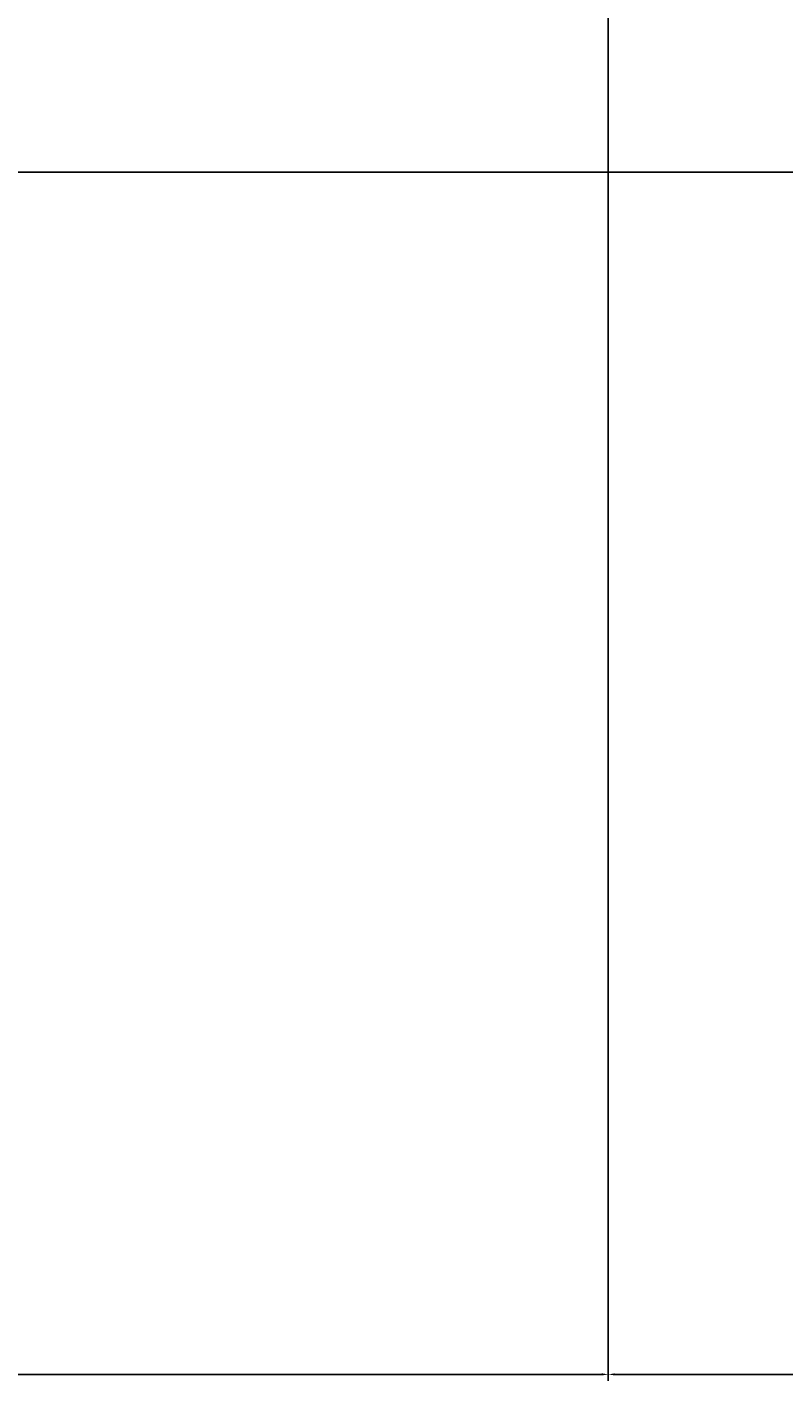
# Model space of a CAD drawing. Units: inches. Extents: x -301 to 715, y -607 to 364.
# Tile 4 of 141: x -3 to 18, y -574 to -536. Entities that reach past the tile are written whole.
import ezdxf

# ---------------------------------------------------------------- set-up
doc = ezdxf.new("R2010")
doc.units = ezdxf.units.IN
doc.header["$MEASUREMENT"] = 0
doc.layers.add('A-ANNO-DIMS', color=2, linetype='Continuous', lineweight=18)
doc.styles.get("Standard").update_dxf_attribs({"font": 'arial.ttf'})
doc.dimstyles.get("Standard").update_dxf_attribs({"dimtxt": 0.18, "dimasz": 0.18, "dimexe": 0.18, "dimexo": 0.0625, "dimgap": 0.09, "dimtad": 0, "dimtih": 1, "dimtoh": 1, "dimdec": 1, "dimzin": 0, "dimdsep": 46, "dimlunit": 4, "dimtxsty": 'Standard', "dimcen": 0.09, "dimclrd": 3, "dimclre": 4, "dimclrt": 6, "dimadec": 0, "dimazin": 0, "dimtfac": 1, "dimtdec": 1, "dimtofl": 0, "dimtmove": 0, "dimatfit": 3, "dimfxl": 1, "dimtfill": 2, "dimtfillclr": 51, "dimtolj": 1, "dimtzin": 0, "dimarcsym": 0})

# ---------------------------------------------------------------- blocks, each defined once
blk = doc.blocks.new('*D176')
at = {"layer": 'A-ANNO-DIMS', "color": 4, "lineweight": -2, "transparency": 16777216}
for p, q in [((148.28, -324.477), (215.605, -324.477)), ((-15.22, -540.477), (215.605, -540.477))]:
    blk.add_line(p, q, dxfattribs=at)
at = {"layer": 'A-ANNO-DIMS', "color": 3, "lineweight": -2, "transparency": 16777216}
for p, q in [((215.425, -324.657), (215.425, -432.296)), ((215.425, -540.297), (215.425, -432.659))]:
    blk.add_line(p, q, dxfattribs=at)
at = {"layer": 'A-ANNO-DIMS', "color": 3, "transparency": 16777216}
for points in [[(215.395, -324.657), (215.455, -324.657), (215.425, -324.477)], [(215.395, -540.297), (215.455, -540.297), (215.425, -540.477)]]:
    blk.add_solid(points, dxfattribs=at)
at = {"layer": 'Defpoints', "color": 0, "transparency": 16777216}
for p in [(148.218, -324.477), (-15.282, -540.477), (215.425, -540.477)]:
    blk.add_point(p, dxfattribs=at)
at = {"layer": 'A-ANNO-DIMS', "color": 6, "transparency": 16777216, "insert": (215.425, -432.477), "char_height": 0.18, "attachment_point": 5, "bg_fill": 1, "box_fill_scale": 1.25, "bg_fill_color": 51, "bg_fill_transparency": 0}
blk.add_mtext('\\A1;18\'-0"', dxfattribs=at)
blk = doc.blocks.new('*D180')
at = {"layer": 'A-ANNO-DIMS', "color": 4, "lineweight": -2, "transparency": 16777216}
for p, q in [((-35.282, -463.54), (-35.282, -573.809)), ((12.718, -463.54), (12.718, -573.809))]:
    blk.add_line(p, q, dxfattribs=at)
at = {"layer": 'A-ANNO-DIMS', "color": 3, "lineweight": -2, "transparency": 16777216}
for p, q in [((-35.102, -573.629), (-11.615, -573.629)), ((12.538, -573.629), (-10.949, -573.629))]:
    blk.add_line(p, q, dxfattribs=at)
at = {"layer": 'A-ANNO-DIMS', "color": 3, "transparency": 16777216}
for points in [[(-35.102, -573.599), (-35.102, -573.659), (-35.282, -573.629)], [(12.538, -573.599), (12.538, -573.659), (12.718, -573.629)]]:
    blk.add_solid(points, dxfattribs=at)
at = {"layer": 'Defpoints', "color": 0, "transparency": 16777216}
for p in [(-35.282, -463.477), (12.718, -463.477), (12.718, -573.629)]:
    blk.add_point(p, dxfattribs=at)
at = {"layer": 'A-ANNO-DIMS', "color": 6, "transparency": 16777216, "insert": (-11.282, -573.629), "char_height": 0.18, "attachment_point": 5, "bg_fill": 1, "box_fill_scale": 1.25, "bg_fill_color": 51, "bg_fill_transparency": 0}
blk.add_mtext('\\A1;4\'-0"', dxfattribs=at)
blk = doc.blocks.new('*D181')
at = {"layer": 'A-ANNO-DIMS', "color": 4, "lineweight": -2, "transparency": 16777216}
for p, q in [((48.468, -433.54), (48.468, -573.809)), ((12.718, -463.54), (12.718, -573.809))]:
    blk.add_line(p, q, dxfattribs=at)
at = {"layer": 'A-ANNO-DIMS', "color": 3, "lineweight": -2, "transparency": 16777216}
for p, q in [((12.898, -573.629), (30.264, -573.629)), ((48.288, -573.629), (30.922, -573.629))]:
    blk.add_line(p, q, dxfattribs=at)
at = {"layer": 'A-ANNO-DIMS', "color": 3, "transparency": 16777216}
for points in [[(12.898, -573.599), (12.898, -573.659), (12.718, -573.629)], [(48.288, -573.599), (48.288, -573.659), (48.468, -573.629)]]:
    blk.add_solid(points, dxfattribs=at)
at = {"layer": 'Defpoints', "color": 0, "transparency": 16777216}
for p in [(48.468, -433.477), (12.718, -463.477), (48.468, -573.629)]:
    blk.add_point(p, dxfattribs=at)
at = {"layer": 'A-ANNO-DIMS', "color": 6, "transparency": 16777216, "insert": (30.593, -573.629), "char_height": 0.18, "attachment_point": 5, "bg_fill": 1, "box_fill_scale": 1.25, "bg_fill_color": 51, "bg_fill_transparency": 0}
blk.add_mtext('\\A1;3\'-0"', dxfattribs=at)
blk = doc.blocks.new('*D191')
at = {"layer": 'A-ANNO-DIMS', "color": 4, "lineweight": -2, "transparency": 16777216}
for p, q in [((129.193, -481.477), (-266.112, -481.477)), ((114.193, -540.477), (-266.112, -540.477))]:
    blk.add_line(p, q, dxfattribs=at)
at = {"layer": 'A-ANNO-DIMS', "color": 3, "lineweight": -2, "transparency": 16777216}
for p, q in [((-265.932, -481.657), (-265.932, -510.797)), ((-265.932, -540.297), (-265.932, -511.158))]:
    blk.add_line(p, q, dxfattribs=at)
at = {"layer": 'A-ANNO-DIMS', "color": 3, "transparency": 16777216}
for points in [[(-265.962, -481.657), (-265.902, -481.657), (-265.932, -481.477)], [(-265.962, -540.297), (-265.902, -540.297), (-265.932, -540.477)]]:
    blk.add_solid(points, dxfattribs=at)
at = {"layer": 'Defpoints', "color": 0, "transparency": 16777216}
for p in [(129.255, -481.477), (-265.932, -540.477), (114.255, -540.477)]:
    blk.add_point(p, dxfattribs=at)
at = {"layer": 'A-ANNO-DIMS', "color": 6, "transparency": 16777216, "insert": (-265.932, -510.977), "char_height": 0.18, "attachment_point": 5, "bg_fill": 1, "box_fill_scale": 1.25, "bg_fill_color": 51, "bg_fill_transparency": 0}
blk.add_mtext('\\A1;4\'-11"', dxfattribs=at)

msp = doc.modelspace()

# ---------------------------------------------------------------- dimensions: what is measured, and where the dimension line sits
at = {"layer": 'A-ANNO-DIMS'}
for base, p1, p2, picture, middle in [((215.425, -540.477), (148.218, -324.477), (-15.282, -540.477), '*D176', (215.425, -432.477)), ((-265.932, -540.477), (129.255, -481.477), (114.255, -540.477), '*D191', (-265.932, -510.977))]:
    dim = msp.add_linear_dim(base=base, p1=p1, p2=p2, angle=90, dimstyle='Standard', override={"dimdec": 1, "dimlfac": 1, "dimrnd": 0, "dimzin": 1, "dimdsep": 46, "dimlunit": 4, "dimfrac": 2}, dxfattribs=at)
    dim.commit()
    dim.dimension.update_dxf_attribs({"geometry": picture, "text_midpoint": middle})
for base, p1, p2, picture, middle in [((48.467984, -573.628877), (12.717984, -463.47741), (48.467984, -433.47741), '*D181', (30.592984, -573.628877)), ((12.718, -573.629), (-35.282, -463.477), (12.718, -463.477), '*D180', (-11.282, -573.629))]:
    dim = msp.add_linear_dim(base=base, p1=p1, p2=p2, dimstyle='Standard', override={"dimdec": 1, "dimlfac": 1, "dimrnd": 0, "dimzin": 1, "dimdsep": 46, "dimlunit": 4, "dimfrac": 2}, dxfattribs=at)
    dim.commit()
    dim.dimension.update_dxf_attribs({"geometry": picture, "text_midpoint": middle})

doc.saveas('drawing.dxf')
